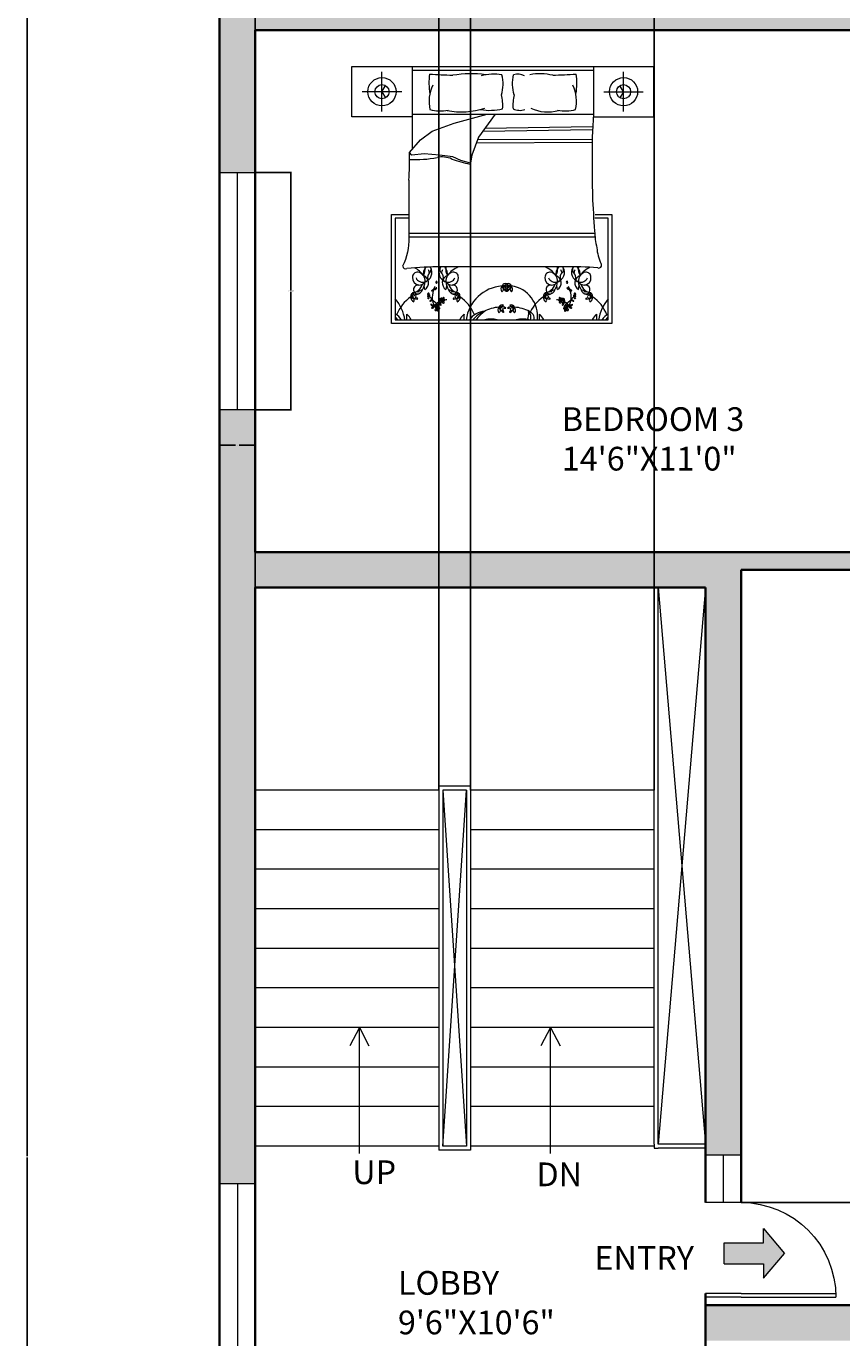
# Model space of a CAD drawing. Units: inches. Extents: x -26 to 13070, y -956 to 6917.
# Tile 6 of 13: x -26 to 180, y -466 to -134. Entities that reach past the tile are written whole.
import ezdxf

# ---------------------------------------------------------------- set-up
doc = ezdxf.new("R2010")
doc.units = ezdxf.units.IN
doc.header["$MEASUREMENT"] = 0
for name, color, linetype, lineweight in [('A-ANNO-DIMS', 2, 'Continuous', 18), ('A-ANNO-SYMB', 7, 'Continuous', 18), ('A-ANNO-TEXT', 7, 'Continuous', 18), ('A-AREA-IDEN', 7, 'Continuous', 18), ('A-DOOR', 3, 'Continuous', 18), ('A-FLOR-STRS', 7, 'Continuous', 18), ('A-FURN', 8, 'Continuous', 13), ('A-GLAZ', 4, 'Continuous', 18), ('A-WALL', 7, 'Continuous', 35), ('A-WALL-PATT', 252, 'Continuous', 13)]:
    doc.layers.add(name, color=color, linetype=linetype, lineweight=lineweight)
doc.styles.get("Standard").update_dxf_attribs({"font": 'arial.ttf'})
doc.dimstyles.get("Standard").update_dxf_attribs({"dimtxt": 0.18, "dimasz": 0.18, "dimexe": 0.18, "dimexo": 0.0625, "dimgap": 0.09, "dimtad": 0, "dimtih": 1, "dimtoh": 1, "dimdec": 0, "dimzin": 0, "dimdsep": 46, "dimlunit": 3, "dimtxsty": 'Standard', "dimcen": 0.09, "dimadec": 0, "dimazin": 0, "dimtfac": 1, "dimtdec": 0, "dimtofl": 0, "dimtmove": 0, "dimatfit": 3, "dimfxl": 1, "dimtolj": 1, "dimtzin": 0, "dimarcsym": 0})

# ---------------------------------------------------------------- blocks, each defined once
blk = doc.blocks.new('BED-DOUBLE-NIGHTSTANDS')
for p, q in [((0, 65), (76.43, 65)), ((7.64, 53.64), (7.64, 63.62)), ((15.29, 65), (15.29, 44.02)), ((61.14, 64.02), (15.29, 64.02)), ((68.79, 53.64), (68.79, 63.62)), ((12.64, 58.63), (2.65, 58.63)), ((63.79, 58.63), (73.78, 58.63)), ((15.29, 52.92), (61.14, 52.92)), ((20.33, 48.64), (25.9, 50.65)), ((25.9, 50.65), (34.24, 52.92)), ((36.28, 52.92), (32.09, 47.09)), ((14.6, 43.22), (17.39, 46.47)), ((17.39, 46.47), (20.33, 48.64)), ((32.09, 47.09), (30.39, 42.6)), ((60.87, 46.55), (31.85, 46.44)), ((60.91, 48.96), (33.16, 48.57)), ((60.94, 49.74), (33.73, 49.36)), ((15.22, 42.6), (14.6, 43.22)), ((60.87, 45.77), (31.55, 45.65)), ((18.32, 42.91), (15.22, 42.6)), ((22.19, 42.6), (18.32, 42.91)), ((25.59, 42.14), (22.19, 42.6)), ((27.6, 41.21), (25.59, 42.14)), ((30.08, 40.59), (27.6, 41.21)), ((30.39, 42.6), (30.08, 40.59)), ((10.09, 27.53), (14.41, 27.53)), ((10.09, 0), (10.09, 27.53)), ((14.41, 26.65), (10.97, 26.65)), ((10.97, 26.65), (10.97, 0.89)), ((64.92, 26.65), (61.55, 26.65)), ((61.57, 27.53), (65.81, 27.53)), ((64.92, 0.89), (64.92, 26.65)), ((65.81, 27.53), (65.81, 0)), ((61.56, 21.81), (14.4, 21.81)), ((61.49, 22.77), (14.41, 22.77)), ((53.73, 14.3), (22.7, 14.3)), ((18.51, 8.63), (18.34, 9.5)), ((23.85, 8.63), (24.02, 9.5)), ((52.05, 8.63), (51.88, 9.5)), ((57.39, 8.63), (57.56, 9.5)), ((10.97, 0.89), (64.92, 0.89)), ((65.81, 0), (10.09, 0))]:
    blk.add_line(p, q)
for points in [[(15.29, 52.26), (0, 52.26), (0, 65)], [(61.14, 65), (61.14, 52.26), (76.43, 52.26), (76.43, 65)], [(7.64, 58.63), (8.53, 60.17)], [(68.79, 58.63), (67.89, 60.17)], [(7.64, 58.63), (8.53, 57.08)], [(68.79, 58.63), (67.89, 57.08)]]:
    blk.add_lwpolyline(points)
for points in [[(19.68, 63.09, 0.074897), (19.77, 58.1, -0.472817)], [(56.75, 63.09, -0.074897), (56.66, 58.1, 0.472817)], [(37.86, 57.82, 0.14099), (38.01, 62.91, 0.235245)], [(41.12, 57.82, -0.14099), (40.97, 62.91, -0.235245)], [(14.44, 36.22, 0.001242), (14.4, 21.72, -0.127202), (12.87, 14.5)], [(61.47, 23.37, 0.056112), (62.02, 19.16, 0.095341), (63.1, 15.11)]]:
    blk.add_lwpolyline(points, format="xyb")
for centre, radius in [((7.64, 58.63), 3.57), ((7.64, 58.63), 1.78), ((68.79, 58.63), 3.57), ((68.79, 58.63), 1.78), ((21.65, 3.81), 0.195), ((22.92, 5.86), 0.195), ((52.98, 5.86), 0.195), ((54.25, 3.81), 0.195)]:
    blk.add_circle(centre, radius)
for centre, radius, start, end in [((61.8, 790.45), 728.57, 266.68521, 267.14978), ((30.15, 35.44), 27.72, 82.2196, 99.497), ((36, 49.44), 13.62, 81.5249, 103.96), ((42.02, 59.28), 3.78, 63.3437, 106.1026), ((47.68, 49.72), 13.44, 76.3427, 101.1841), ((14.63, 790.45), 728.57, 272.85022, 273.31479), ((29.41, 56.1), 9.85, 155.1316, 191.7583), ((47.02, 56.1), 9.85, 348.2417, 24.8684), ((28.85, 55.27), 9.36, 354.0129, 15.8293), ((50.13, 55.27), 9.36, 164.1707, 185.9871), ((22.4, 63.99), 10.24, 255.1039, 281.0369), ((27.79, 71.27), 17.76, 258.0397, 289.2615), ((34.99, 67.39), 13.48, 259.8617, 283.6238), ((42.53, 57.96), 4.05, 245.0183, 288.5407), ((49.61, 63.23), 9.73, 243.8761, 286.1746), ((54.03, 63.99), 10.24, 258.9631, 284.8961), ((198.16, 43.58), 137.33, 176.1, 180.9282), ((-55.48, 41.32), 70.1, 355.8294, 1.553), ((15.91, 70.29), 28.85, 267.4519, 281.3392), ((22.8, 35.91), 6.22, 66.2616, 101.3392), ((35.39, 69.47), 29.64, 250.1194, 259.3383), ((29.91, 40.53), 0.184, 268.8623, 19.7536), ((239.96, 38.59), 179.14, 179.1145, 184.8735), ((13.58, 14.54), 0.705, 183.98, 297.3412), ((21.79, -65.25), 79.56, 89.3433, 95.6887), ((13.28, 8.92), 5.78, 33.6671, 63.2997), ((21.03, 12.36), 2.95, 145.785, 184.7304), ((15.4, 13.74), 3.17, 328.8218, 9.1554), ((19.32, 13.46), 0.92, 120.0293, 142.325), ((17.85, 12.92), 2.44, 289.2822, 29.1751), ((17.48, 12.48), 2.2, 7.436, 29.9149), ((18.93, 13.64), 1.14, 311.5653, 23.8354), ((19.32, 13.46), 0.92, 44.4517, 63.558), ((24.5, 12.92), 2.44, 150.8249, 250.7178), ((23.42, 13.64), 1.14, 156.1646, 228.4347), ((23.03, 13.46), 0.92, 113.229, 135.5483), ((24.87, 12.48), 2.2, 150.0851, 172.564), ((23.03, 13.46), 0.92, 37.675, 66.7144), ((21.32, 12.36), 2.95, 355.2696, 34.215), ((26.95, 13.74), 3.17, 169.7133, 211.1782), ((29.07, 8.92), 5.78, 111.4941, 146.3329), ((46.82, 8.92), 5.78, 33.6671, 68.5059), ((54.57, 12.36), 2.95, 145.785, 184.7304), ((48.94, 13.74), 3.17, 328.8218, 10.2867), ((52.87, 13.46), 0.92, 113.2856, 142.325), ((51.4, 12.92), 2.44, 289.2822, 29.1751), ((51.03, 12.48), 2.2, 7.436, 29.9149), ((52.87, 13.46), 0.92, 44.4517, 66.7144), ((52.48, 13.64), 1.14, 311.5653, 23.8354), ((56.07, -60.03), 74.37, 85.2402, 91.8035), ((58.04, 12.92), 2.44, 150.8249, 250.7178), ((56.96, 13.64), 1.14, 156.1646, 228.4347), ((56.57, 13.46), 0.92, 106.6343, 135.5483), ((58.41, 12.48), 2.2, 150.0851, 172.564), ((56.57, 13.46), 0.92, 37.675, 72.5814), ((54.87, 12.36), 2.95, 355.2696, 34.215), ((60.5, 13.74), 3.17, 169.249, 211.1782), ((62.62, 8.92), 5.78, 113.6453, 146.3329), ((62.52, 14.72), 0.697, 246.5219, 33.8264), ((17.18, 11.52), 1.83, 174.9449, 262.8857), ((16.65, 11.7), 1.29, 84.4856, 181.0538), ((17.9, 12.21), 1.77, 201.5819, 291.4221), ((14.48, 11.1), 3.61, 301.2614, 341.7045), ((16.25, 10.75), 2.3, 355.2933, 76.921), ((16.86, 11.92), 2.22, 272.3591, 324.0401), ((14.45, 10.81), 4.1, 326.2883, 356.5076), ((17.56, 10.28), 1.9, 299.9085, 73.1337), ((21.03, 12.36), 2.95, 212.7011, 216.3445), ((18.76, 11.08), 0.474, 257.3041, 15.1471), ((20.73, 11.61), 1.57, 131.5653, 195.1471), ((21.4, 10.36), 0.147, 102.7051, 280.4384), ((21.38, 10.45), 0.24, 280.4384, 100.4136), ((21.62, 11.61), 1.57, 344.8529, 48.4347), ((24.79, 10.28), 1.9, 106.8663, 240.0915), ((23.59, 11.08), 0.474, 164.8529, 282.6959), ((21.32, 12.36), 2.95, 323.6555, 327.2989), ((25.49, 11.92), 2.22, 215.9599, 267.6409), ((26.1, 10.75), 2.3, 103.079, 184.7067), ((24.46, 12.21), 1.77, 248.5779, 338.4181), ((27.9, 10.81), 4.1, 183.4924, 213.7117), ((27.87, 11.1), 3.61, 198.2955, 238.7386), ((25.17, 11.52), 1.83, 277.1143, 5.0551), ((25.7, 11.7), 1.29, 358.9462, 95.5144), ((38.83, 9.26), 0.827, 63.0274, 163.8037), ((37.99, 11.2), 1.7, 271.4585, 315.3727), ((39.62, 9.26), 0.827, 16.1963, 116.9726), ((40.45, 11.2), 1.7, 224.6273, 268.5415), ((50.72, 11.52), 1.83, 174.9449, 262.8857), ((50.19, 11.7), 1.29, 84.4856, 181.0538), ((51.44, 12.21), 1.77, 201.5819, 291.4221), ((48.03, 11.1), 3.61, 301.2614, 341.7045), ((49.8, 10.75), 2.3, 355.2933, 76.921), ((50.4, 11.92), 2.22, 272.3591, 324.0401), ((47.99, 10.81), 4.1, 326.2883, 356.5076), ((51.1, 10.28), 1.9, 299.9085, 73.1337), ((54.57, 12.36), 2.95, 212.7011, 216.3445), ((52.3, 11.08), 0.474, 257.3041, 15.1471), ((54.28, 11.61), 1.57, 131.5653, 195.1471), ((54.52, 10.45), 0.24, 79.5864, 259.5616), ((54.5, 10.36), 0.147, 259.5616, 77.2949), ((55.16, 11.61), 1.57, 344.8529, 48.4347), ((58.34, 10.28), 1.9, 106.8663, 240.0915), ((57.13, 11.08), 0.474, 164.8529, 282.6959), ((54.87, 12.36), 2.95, 323.6555, 327.2989), ((59.04, 11.92), 2.22, 215.9599, 267.6409), ((59.64, 10.75), 2.3, 103.079, 184.7067), ((58, 12.21), 1.77, 248.5779, 338.4181), ((61.45, 10.81), 4.1, 183.4924, 213.7117), ((61.41, 11.1), 3.61, 198.2955, 238.7386), ((58.72, 11.52), 1.83, 277.1143, 5.0551), ((59.25, 11.7), 1.29, 358.9462, 95.5144), ((20.62, -1.45), 9.98, 124.3865, 158.5908), ((15.79, 6.99), 0.827, 92.9516, 193.728), ((16.06, 6.55), 1.11, 167.7115, 249.0387), ((14.09, 8.25), 1.7, 301.3827, 345.2969), ((16.26, 5.87), 1.58, 75.4653, 144.2343), ((13.47, 13.61), 6.98, 282.5173, 297.1824), ((14.96, 5.96), 0.834, 328.4633, 88.2869), ((16.64, 8.69), 2.52, 228.8402, 267.9352), ((15.7, 7.17), 0.816, 207.6827, 313.7762), ((16.76, 8.57), 1.15, 80.264, 250.8688), ((16.52, 7.33), 0.703, 63.9755, 143.2681), ((16.19, 6.66), 0.108, 313.7762, 249.7183), ((16.48, 8.92), 1.43, 265.969, 344.3045), ((18.02, 7.01), 1.53, 96.1662, 141.5825), ((19.42, 7.32), 0.325, 101.5637, 142.6358), ((19.15, 7.02), 0.195, 273.2768, 86.7232), ((19.37, 7.21), 0.186, 91.1081, 181.8675), ((19.76, 7.09), 0.591, 203.4276, 227.6104), ((19.57, 6.83), 0.402, 80.3487, 133.6538), ((19.5, 7.16), 0.318, 229.7889, 317.6792), ((19.16, 7.58), 0.468, 288.7263, 352.5032), ((19.14, 6.49), 0.452, 355.053, 68.3618), ((19.5, 6.41), 0.637, 83.0852, 105.7171), ((19.47, 7.55), 0.15, 345.2356, 144.9248), ((15.08, 1.13), 7.26, 43.1541, 52.0459), ((19.61, 7.06), 0.168, 317.6792, 80.3487), ((20.55, 8.08), 0.401, 101.3256, 154.4621), ((19.97, 9.45), 1.21, 280.2588, 300.656), ((20.25, 10.41), 2.16, 268.3264, 277.1302), ((26.69, 6.51), 6.33, 163.5842, 183.8277), ((19.71, 9.44), 1.23, 308.2101, 316.3071), ((20.47, 8.64), 0.367, 278.3432, 4.2869), ((20.26, 8.96), 0.641, 300.656, 332.6341), ((20.74, 8.53), 0.156, 55.7657, 157.4417), ((26.69, 6.51), 6.33, 153.0032, 159.8941), ((20.99, 8.68), 0.156, 84.3784, 186.0543), ((20.84, 9.3), 0.641, 269.1859, 301.164), ((21.03, 8.97), 0.367, 237.5332, 323.4768), ((20.67, 10.02), 1.23, 285.5129, 293.6099), ((20.55, 9.79), 1.21, 301.164, 321.5612), ((21.48, 8.64), 0.401, 87.3579, 140.4944), ((19.56, 10), 2.16, 324.6898, 333.4936), ((24.33, 7.01), 1.53, 38.4175, 83.8338), ((25.87, 8.92), 1.43, 195.6955, 274.031), ((25.59, 8.57), 1.15, 289.1312, 99.736), ((25.83, 7.33), 0.703, 36.7319, 116.0245), ((26.09, 5.87), 1.58, 35.7657, 104.5347), ((28.88, 13.61), 6.98, 242.8176, 257.4827), ((25.71, 8.69), 2.52, 272.0648, 311.1598), ((26.65, 7.17), 0.816, 226.2238, 332.3173), ((26.17, 6.7), 0.0651, 290.2667, 226.2271), ((27.4, 5.96), 0.834, 91.7131, 211.5367), ((26.57, 6.99), 0.827, 346.272, 87.0484), ((28.26, 8.25), 1.7, 194.7031, 238.6173), ((26.29, 6.55), 1.11, 290.9613, 12.2885), ((21.73, -1.45), 9.98, 21.4092, 55.6135), ((38.81, -0.46), 9.98, 94.4623, 172.255), ((38.85, 8.75), 1.11, 137.7873, 219.1145), ((37.6, 8.78), 0.834, 298.5391, 58.3627), ((38.68, 8.05), 1.58, 45.5411, 114.3101), ((40.12, 16.15), 6.98, 252.593, 267.2582), ((38.85, 9.46), 0.816, 177.7585, 283.852), ((40.42, 10.31), 2.52, 198.9159, 238.011), ((39.76, 8.05), 1.58, 65.6899, 134.4589), ((38.32, 16.15), 6.98, 272.7418, 287.407), ((39.02, 8.77), 0.108, 283.852, 219.9245), ((39.15, 8.27), 0.124, 238.011, 71.5592), ((39.17, 8.33), 0.0602, 71.5592, 188.0167), ((39.29, 8.27), 0.124, 108.4408, 301.989), ((39.27, 8.33), 0.0602, 351.9833, 108.4408), ((39.42, 8.81), 0.0651, 320.1909, 256.0209), ((38.02, 10.31), 2.52, 301.989, 341.0841), ((39.6, 9.46), 0.816, 256.148, 2.2415), ((40.85, 8.78), 0.834, 121.6373, 241.4609), ((39.59, 8.75), 1.11, 320.8855, 42.2127), ((39.31, 1.85), 7.72, 352.8636, 81.8197), ((54.16, -1.45), 9.98, 124.3865, 158.5908), ((49.33, 6.99), 0.827, 92.9516, 193.728), ((49.61, 6.55), 1.11, 167.7115, 249.0387), ((47.64, 8.25), 1.7, 301.3827, 345.2969), ((49.81, 5.87), 1.58, 75.4653, 144.2343), ((47.01, 13.61), 6.98, 282.5173, 297.1824), ((49.25, 7.17), 0.816, 207.6827, 313.7762), ((50.19, 8.69), 2.52, 228.8402, 267.9352), ((48.5, 5.96), 0.834, 328.4633, 88.2869), ((50.3, 8.57), 1.15, 80.264, 250.8688), ((50.06, 7.33), 0.703, 63.9755, 143.2681), ((49.74, 6.66), 0.108, 313.7762, 249.7183), ((50.03, 8.92), 1.43, 265.969, 344.3045), ((51.57, 7.01), 1.53, 96.1662, 141.5825), ((55.35, 9.79), 1.21, 218.4388, 238.836), ((54.42, 8.64), 0.401, 39.5056, 92.6421), ((56.33, 10), 2.16, 206.5064, 215.3102), ((54.87, 8.97), 0.367, 216.5232, 302.4668), ((55.05, 9.3), 0.641, 238.836, 270.8141), ((55.22, 10.02), 1.23, 246.3901, 254.4871), ((49.2, 6.51), 6.33, 20.1059, 26.9968), ((54.91, 8.68), 0.156, 353.9457, 95.6216), ((55.15, 8.53), 0.156, 22.5583, 124.2343), ((55.43, 8.64), 0.367, 175.7131, 261.6568), ((55.63, 8.96), 0.641, 207.3659, 239.344), ((49.2, 6.51), 6.33, 356.1723, 16.4158), ((56.18, 9.44), 1.23, 223.6929, 231.7899), ((55.92, 9.45), 1.21, 239.344, 259.7412), ((55.64, 10.41), 2.16, 262.8698, 271.6736), ((55.34, 8.08), 0.401, 25.5379, 78.6744), ((60.81, 1.13), 7.26, 127.9541, 136.8459), ((56.28, 7.06), 0.168, 99.6513, 222.3208), ((56.4, 7.16), 0.318, 222.3208, 310.2111), ((56.32, 6.83), 0.402, 46.3462, 99.6513), ((56.42, 7.55), 0.15, 35.0752, 194.7644), ((56.74, 7.58), 0.468, 187.4968, 251.2737), ((56.76, 6.49), 0.452, 111.6382, 184.947), ((56.4, 6.41), 0.637, 74.2829, 96.9148), ((56.52, 7.21), 0.186, 358.1325, 88.8919), ((56.14, 7.09), 0.591, 312.3896, 336.5724), ((56.48, 7.32), 0.325, 37.3642, 78.4363), ((56.75, 7.02), 0.195, 93.2768, 266.7232), ((59.41, 8.92), 1.43, 195.6955, 274.031), ((57.87, 7.01), 1.53, 38.4175, 83.8338), ((59.14, 8.57), 1.15, 289.1312, 99.736), ((59.37, 7.33), 0.703, 36.7319, 116.0245), ((59.63, 5.87), 1.58, 35.7657, 104.5347), ((62.43, 13.61), 6.98, 242.8176, 257.4827), ((59.25, 8.69), 2.52, 272.0648, 311.1598), ((60.19, 7.17), 0.816, 226.2238, 332.3173), ((59.71, 6.7), 0.0651, 290.2667, 226.2271), ((60.94, 5.96), 0.834, 91.7131, 211.5367), ((61.8, 8.25), 1.7, 194.7031, 238.6173), ((60.11, 6.99), 0.827, 346.272, 87.0484), ((59.83, 6.55), 1.11, 290.9613, 12.2885), ((55.28, -1.45), 9.98, 21.4092, 55.6135), ((3.54, -0.46), 9.98, 7.745, 41.8856), ((16.54, 6.35), 0.0602, 101.4834, 217.9409), ((16.56, 6.29), 0.124, 267.9352, 101.4834), ((19.41, 6.66), 0.321, 217.7621, 259.0403), ((19.44, 6.46), 0.149, 232.4737, 355.053), ((20.1, 5.51), 0.401, 101.3256, 154.4621), ((19.52, 6.87), 1.21, 280.2588, 300.656), ((19.8, 7.84), 2.16, 268.3264, 277.1302), ((20.23, 4.81), 0.217, 146.8636, 236.9021), ((19.26, 6.87), 1.23, 308.2101, 316.3071), ((23.3, 9.6), 5.69, 235.1882, 238.8844), ((20.6, 5.12), 0.588, 199.4799, 267.6828), ((20.01, 6.06), 0.367, 278.3432, 4.2869), ((20.54, 4.9), 0.507, 212.8155, 277.3992), ((19.81, 6.39), 0.641, 300.656, 332.6341), ((20.29, 5.96), 0.156, 55.7657, 157.4417), ((20.24, 4.56), 0.588, 266.9701, 338.2913), ((17.14, 8.76), 5.69, 302.6784, 306.3746), ((20.39, 4.1), 0.217, 214.3538, 304.3923), ((20.47, 4.92), 0.225, 238.8844, 314.2646), ((23.54, 6.35), 3.17, 184.756, 209.2041), ((28.11, 13.11), 10.44, 222.2412, 232.1744), ((20.42, 4.42), 0.507, 280.3057, 17.1958), ((20.38, 4.36), 0.225, 306.3746, 21.7548), ((20.75, 4.51), 0.17, 19.3605, 201.7548), ((20.75, 4.64), 0.17, 311.8703, 134.2646), ((23.94, 3.09), 3.39, 153.7819, 158.2913), ((21.24, 5.41), 0.887, 247.2305, 319.0635), ((20.95, 5.11), 0.522, 264.4544, 310.6188), ((23.54, 6.35), 3.17, 214.0033, 222.4917), ((21.33, 4.9), 0.539, 218.3208, 298.8162), ((23.87, 2.14), 3.81, 120.544, 139.818), ((21.24, 3.45), 0.193, 148.0499, 225.6268), ((21.6, 3.23), 0.614, 104.7558, 148.0499), ((21.25, 3.66), 0.384, 247.4086, 351.4386), ((21.43, 4.08), 0.265, 126.1046, 271.4281), ((21.4, 4.16), 0.191, 353.7526, 131.7054), ((21.7, 4.23), 0.628, 70.0041, 130.6188), ((21.36, 3.65), 0.129, 262.906, 7.132), ((21.22, 3.93), 0.268, 0.0645, 61.1507), ((21.29, 4.16), 0.306, 311.8413, 355.7877), ((21.29, 5), 0.645, 297.7043, 344.3516), ((21.92, 4.11), 0.325, 101.5637, 176.365), ((21.91, 3.45), 0.321, 151.2196, 259.0403), ((21.87, 4), 0.186, 91.1081, 181.8675), ((22.26, 3.88), 0.591, 203.4276, 227.6104), ((22.07, 3.62), 0.402, 80.3487, 133.6538), ((22, 3.96), 0.318, 229.7889, 317.6792), ((21.66, 4.37), 0.468, 288.7263, 352.5032), ((21.64, 3.28), 0.452, 355.053, 68.3618), ((22, 3.21), 0.637, 83.0852, 105.7171), ((21.97, 4.35), 0.15, 345.2356, 144.9248), ((21.43, 6.15), 0.887, 304.5369, 16.3699), ((21.9, 5.96), 0.539, 272.8499, 356.1226), ((21.52, 5.75), 0.522, 321.7607, 7.9252), ((21.63, 5), 0.522, 8.7227, 54.8872), ((21.66, 4.58), 0.887, 0.278, 72.111), ((22.66, 5.9), 0.628, 127.3105, 187.9252), ((22.06, 4.9), 0.539, 20.5253, 88.5375), ((22.11, 3.85), 0.168, 317.6792, 80.3487), ((22.77, 5.17), 0.628, 188.7227, 249.3375), ((21.8, 5.98), 0.645, 355.0106, 41.658), ((22.51, 5.5), 0.193, 148.0499, 225.6268), ((23.87, 2.14), 3.81, 113.0501, 113.8477), ((22.87, 5.28), 0.614, 104.7558, 148.0499), ((22.52, 5.72), 0.384, 247.4086, 351.4386), ((22.71, 6.14), 0.265, 126.1046, 271.4281), ((22.68, 6.21), 0.191, 353.7526, 131.7054), ((21.96, 4.86), 0.645, 334.9899, 21.6373), ((22.63, 5.7), 0.129, 262.906, 7.132), ((22.5, 5.98), 0.268, 0.0645, 61.1507), ((22.56, 6.21), 0.306, 311.8413, 355.7877), ((23.19, 5.5), 0.321, 151.2196, 259.0403), ((23.19, 6.17), 0.325, 101.5637, 176.365), ((23.15, 6.05), 0.186, 91.1081, 181.8675), ((23.53, 5.93), 0.591, 203.4276, 227.6104), ((23.35, 5.67), 0.402, 80.3487, 133.6538), ((23.27, 6.01), 0.318, 229.7889, 317.6792), ((22.93, 6.42), 0.468, 288.7263, 352.5032), ((22.91, 5.33), 0.452, 355.053, 68.3618), ((23.27, 5.26), 0.637, 83.0852, 105.7171), ((23.25, 6.4), 0.15, 345.2356, 144.9248), ((23.22, 5.31), 0.149, 232.4737, 355.053), ((23.38, 5.91), 0.168, 317.6792, 80.3487), ((23.87, 2.14), 3.81, 87.1071, 94.7585), ((25.8, 6.29), 0.124, 78.5166, 272.0648), ((25.81, 6.35), 0.0602, 322.0591, 78.5166), ((38.04, -5.81), 9.98, 94.4623, 117.4146), ((38.09, 3.4), 1.11, 137.7873, 219.1145), ((36.83, 3.44), 0.834, 298.5391, 58.3627), ((38.06, 3.91), 0.827, 63.0274, 163.8037), ((37.22, 5.85), 1.7, 271.4585, 315.3727), ((37.92, 2.71), 1.58, 45.5411, 114.3101), ((39.66, 4.96), 2.52, 198.9159, 238.011), ((39.36, 10.81), 6.98, 252.593, 267.2582), ((38.08, 4.11), 0.816, 177.7585, 283.852), ((38.25, 3.43), 0.108, 283.852, 219.9245), ((40.53, 2.71), 1.58, 65.6899, 134.4589), ((39.09, 10.81), 6.98, 272.7418, 287.407), ((40.38, 3.91), 0.827, 16.1963, 116.9726), ((41.22, 5.85), 1.7, 224.6273, 268.5415), ((40.18, 3.47), 0.0651, 320.1909, 256.0209), ((38.79, 4.96), 2.52, 301.989, 341.0841), ((40.36, 4.11), 0.816, 256.148, 2.2415), ((41.61, 3.44), 0.834, 121.6373, 241.4609), ((40.36, 3.4), 1.11, 320.8855, 42.2127), ((40.4, -5.81), 9.98, 62.5854, 85.5377), ((50.09, 6.35), 0.0602, 101.4834, 217.9409), ((50.1, 6.29), 0.124, 267.9352, 101.4834), ((52.03, 2.14), 3.81, 85.2415, 92.8929), ((52.51, 5.91), 0.168, 99.6513, 222.3208), ((52.62, 6.01), 0.318, 222.3208, 310.2111), ((52.55, 5.67), 0.402, 46.3462, 99.6513), ((52.65, 6.4), 0.15, 35.0752, 194.7644), ((52.97, 6.42), 0.468, 187.4968, 251.2737), ((52.98, 5.33), 0.452, 111.6382, 184.947), ((52.68, 5.31), 0.149, 184.947, 307.5263), ((52.63, 5.26), 0.637, 74.2829, 96.9148), ((52.75, 6.05), 0.186, 358.1325, 88.8919), ((52.36, 5.93), 0.591, 312.3896, 336.5724), ((52.71, 6.17), 0.325, 3.635, 78.4363), ((52.71, 5.5), 0.321, 280.9597, 28.7804), ((53.37, 5.72), 0.384, 188.5614, 292.5914), ((53.22, 6.21), 0.191, 48.2946, 186.2474), ((53.34, 6.21), 0.306, 184.2123, 228.1587), ((53.4, 5.98), 0.268, 118.8493, 179.9355), ((53.26, 5.7), 0.129, 172.868, 277.094), ((53.19, 6.14), 0.265, 268.5719, 53.8954), ((53.03, 5.28), 0.614, 31.9501, 75.2442), ((53.93, 4.86), 0.645, 158.3627, 205.0101), ((53.84, 4.9), 0.539, 91.4625, 159.4747), ((54.23, 4.58), 0.887, 107.889, 179.722), ((53.13, 5.17), 0.628, 290.6625, 351.2773), ((54.1, 5.98), 0.645, 138.342, 184.9894), ((53.99, 5.96), 0.539, 183.8774, 267.1501), ((52.03, 2.14), 3.81, 66.1523, 66.9499), ((53.38, 5.5), 0.193, 314.3732, 31.9501), ((54.47, 6.15), 0.887, 163.6301, 235.4631), ((53.23, 5.9), 0.628, 352.0748, 52.6895), ((53.78, 3.85), 0.168, 99.6513, 222.3208), ((53.9, 3.96), 0.318, 222.3208, 310.2111), ((54.26, 5), 0.522, 125.1128, 171.2773), ((53.82, 3.62), 0.402, 46.3462, 99.6513), ((53.92, 4.35), 0.15, 35.0752, 194.7644), ((54.24, 4.37), 0.468, 187.4968, 251.2737), ((54.26, 3.28), 0.452, 111.6382, 184.947), ((53.9, 3.21), 0.637, 74.2829, 96.9148), ((54.37, 5.75), 0.522, 172.0748, 218.2393), ((52.03, 2.14), 3.81, 40.182, 59.456), ((54.2, 4.23), 0.628, 49.3812, 109.9959), ((54.65, 5.41), 0.887, 220.9365, 292.7695), ((54.6, 5), 0.645, 195.6484, 242.2957), ((54.02, 4), 0.186, 358.1325, 88.8919), ((53.64, 3.88), 0.591, 312.3896, 336.5724), ((53.98, 4.11), 0.325, 3.635, 78.4363), ((53.98, 3.45), 0.321, 280.9597, 28.7804), ((47.79, 13.11), 10.44, 307.8256, 317.7588), ((54.64, 3.66), 0.384, 188.5614, 292.5914), ((54.56, 4.9), 0.539, 241.1838, 321.6792), ((54.49, 4.16), 0.191, 48.2946, 186.2474), ((54.61, 4.16), 0.306, 184.2123, 228.1587), ((54.67, 3.93), 0.268, 118.8493, 179.9355), ((54.54, 3.65), 0.129, 172.868, 277.094), ((54.46, 4.08), 0.265, 268.5719, 53.8954), ((54.3, 3.23), 0.614, 31.9501, 75.2442), ((54.95, 5.11), 0.522, 229.3812, 275.5456), ((52.36, 6.35), 3.17, 317.5083, 325.9967), ((54.66, 3.45), 0.193, 314.3732, 31.9501), ((55.47, 4.42), 0.507, 162.8042, 259.6943), ((55.15, 4.64), 0.17, 45.7354, 228.1297), ((55.15, 4.51), 0.17, 338.2452, 160.6395), ((51.96, 3.09), 3.39, 21.7087, 26.2181), ((55.65, 4.56), 0.588, 201.7087, 273.0299), ((52.36, 6.35), 3.17, 330.7959, 355.244), ((55.42, 4.92), 0.225, 225.7354, 301.1156), ((55.36, 4.9), 0.507, 262.6008, 327.1845), ((55.51, 4.36), 0.225, 158.2452, 233.6254), ((55.29, 5.12), 0.588, 272.3172, 340.5201), ((58.75, 8.76), 5.69, 233.6254, 237.3216), ((55.5, 4.1), 0.217, 235.6077, 325.6462), ((55.61, 5.96), 0.156, 22.5583, 124.2343), ((55.88, 6.06), 0.367, 175.7131, 261.6568), ((56.09, 6.39), 0.641, 207.3659, 239.344), ((52.6, 9.6), 5.69, 301.1156, 304.8118), ((56.64, 6.87), 1.23, 223.6929, 231.7899), ((56.38, 6.87), 1.21, 239.344, 259.7412), ((55.66, 4.81), 0.217, 303.0979, 33.1364), ((56.1, 7.84), 2.16, 262.8698, 271.6736), ((55.8, 5.51), 0.401, 25.5379, 78.6744), ((56.45, 6.46), 0.149, 184.947, 307.5263), ((56.48, 6.66), 0.321, 280.9597, 322.2379), ((59.34, 6.29), 0.124, 78.5166, 272.0648), ((59.35, 6.35), 0.0602, 322.0591, 78.5166), ((72.35, -0.46), 9.98, 138.1144, 172.255), ((8.55, -1.8), 4.86, 33.4617, 60.1116), ((6.8, -2.7), 6.06, 36.3036, 46.4814), ((11.27, -0.67), 4.06, 22.5547, 48.9546), ((0.16, 1.51), 13.81, 357.4081, 3.6519), ((21.94, 3.26), 0.149, 232.4737, 355.053), ((31.08, -0.67), 4.06, 131.0454, 157.4453), ((42.19, 1.51), 13.81, 176.3481, 182.5919), ((33.8, -1.8), 4.86, 91.272, 146.5383), ((35.55, -2.7), 6.06, 107.8504, 143.6964), ((38.74, -4.41), 9.02, 124.0123, 144.053), ((35.25, -4.36), 5.49, 73.5431, 107.0202), ((37.43, -7.19), 8.12, 94.3787, 95.6357), ((41.7, -12.75), 14.5, 109.7217, 109.9028), ((38.38, 2.93), 0.124, 238.011, 71.5592), ((38.4, 2.99), 0.0602, 71.5592, 188.0167), ((40.06, 2.93), 0.124, 108.4408, 301.989), ((40.04, 2.99), 0.0602, 351.9833, 108.4408), ((43.19, -4.36), 5.49, 72.9798, 106.4569), ((41.02, -7.19), 8.12, 84.3643, 85.6213), ((36.74, -12.75), 14.5, 70.0972, 70.2783), ((40.31, 2.55), 4.47, 338.117, 6.6195), ((44.41, 1.31), 1.79, 346.3898, 79.0739), ((43.06, 1.55), 2.27, 342.8609, 41.9049), ((33.7, 1.51), 13.81, 357.4081, 3.6519), ((44.82, -0.67), 4.06, 22.5547, 48.9546), ((53.95, 3.26), 0.149, 184.947, 307.5263), ((64.62, -0.67), 4.06, 131.0454, 157.4453), ((75.74, 1.51), 13.81, 176.3481, 182.5919), ((67.35, -1.8), 4.86, 119.8884, 146.5383), ((69.1, -2.7), 6.06, 133.5186, 143.6964)]:
    blk.add_arc(centre, radius, start, end)
blk = doc.blocks.new('DOOR-SWING-24')
for p, q in [((24, 1), (0, 1)), ((24, 0), (0, 0))]:
    blk.add_line(p, q)
blk.add_arc((24, 0), 24, 90, 180)
blk = doc.blocks.new('WIN-60')
for p, q in [((0, 0), (0, 60)), ((0, 60), (9, 60)), ((4.5, 0), (4.5, 60)), ((9, 60), (9, 0)), ((9, 0), (0, 0))]:
    blk.add_line(p, q)
blk = doc.blocks.new('STAIR-TRAVEL-ARROW')
for p, q in [((2.41, 31.83), (0, 27.19)), ((2.41, 0), (2.41, 31.83)), ((2.41, 31.83), (4.82, 27.19))]:
    blk.add_line(p, q)
blk = doc.blocks.new('*D20')
at = {"layer": 'A-ANNO-DIMS', "color": 0, "lineweight": -2, "transparency": 16777216}
for p, q in [((31.7, -171.04), (40.82, -171.04)), ((40.64, -171.22), (40.64, -200.86)), ((40.64, -230.86), (40.64, -201.22)), ((31.7, -231.04), (40.82, -231.04))]:
    blk.add_line(p, q, dxfattribs=at)
at = {"layer": 'A-ANNO-DIMS', "color": 0, "transparency": 16777216}
for points in [[(40.61, -171.22), (40.67, -171.22), (40.64, -171.04)], [(40.61, -230.86), (40.67, -230.86), (40.64, -231.04)]]:
    blk.add_solid(points, dxfattribs=at)
at = {"layer": 'Defpoints', "color": 0, "transparency": 16777216}
for p in [(31.64, -171.04), (40.64, -171.04), (31.64, -231.04)]:
    blk.add_point(p, dxfattribs=at)
at = {"layer": 'A-ANNO-DIMS', "color": 0, "transparency": 16777216, "insert": (40.64, -201.04), "char_height": 0.18, "attachment_point": 5}
blk.add_mtext('\\A1;WINDOW 60 TYP.', dxfattribs=at)
blk = doc.blocks.new('*D21')
at = {"layer": 'A-ANNO-DIMS', "color": 0, "lineweight": -2, "transparency": 16777216}
for p, q in [((22.64, -231.1), (22.64, -240.22)), ((31.64, -231.1), (31.64, -240.22)), ((22.82, -240.04), (26.68, -240.04)), ((31.46, -240.04), (27.6, -240.04))]:
    blk.add_line(p, q, dxfattribs=at)
at = {"layer": 'A-ANNO-DIMS', "color": 0, "transparency": 16777216}
for points in [[(22.82, -240.01), (22.82, -240.07), (22.64, -240.04)], [(31.46, -240.01), (31.46, -240.07), (31.64, -240.04)]]:
    blk.add_solid(points, dxfattribs=at)
at = {"layer": 'Defpoints', "color": 0, "transparency": 16777216}
for p in [(22.64, -231.04), (31.64, -231.04), (31.64, -240.04)]:
    blk.add_point(p, dxfattribs=at)
at = {"layer": 'A-ANNO-DIMS', "color": 0, "transparency": 16777216, "insert": (27.14, -240.04), "char_height": 0.18, "attachment_point": 5}
blk.add_mtext('\\A1;9 TYP.', dxfattribs=at)
blk = doc.blocks.new('*D41')
at = {"layer": 'A-ANNO-DIMS', "color": 0, "lineweight": -2, "transparency": 16777216}
for p, q in [((214.58, 67.46), (-26.29, 67.46)), ((-26.11, 67.28), (-26.11, -419.86)), ((-26.11, -907.36), (-26.11, -420.22)), ((208.58, -907.54), (-26.29, -907.54))]:
    blk.add_line(p, q, dxfattribs=at)
at = {"layer": 'A-ANNO-DIMS', "color": 0, "transparency": 16777216}
for points in [[(-26.14, 67.28), (-26.08, 67.28), (-26.11, 67.46)], [(-26.14, -907.36), (-26.08, -907.36), (-26.11, -907.54)]]:
    blk.add_solid(points, dxfattribs=at)
at = {"layer": 'Defpoints', "color": 0, "transparency": 16777216}
for p in [(-26.11, 67.46), (214.64, 67.46), (208.64, -907.54)]:
    blk.add_point(p, dxfattribs=at)
at = {"layer": 'A-ANNO-DIMS', "color": 0, "transparency": 16777216, "insert": (-26.11, -420.04), "char_height": 0.18, "attachment_point": 5}
blk.add_mtext('\\A1;975', dxfattribs=at)
blk = doc.blocks.new('*D55')
at = {"layer": 'A-ANNO-DIMS', "color": 0, "lineweight": -2, "transparency": 16777216}
for p, q in [((31.64, -327.23), (31.64, 116.39)), ((31.82, 116.21), (54.56, 116.21)), ((77.96, 116.21), (55.22, 116.21)), ((78.14, -327.23), (78.14, 116.39))]:
    blk.add_line(p, q, dxfattribs=at)
at = {"layer": 'A-ANNO-DIMS', "color": 0, "transparency": 16777216}
for points in [[(31.82, 116.24), (31.82, 116.18), (31.64, 116.21)], [(77.96, 116.24), (77.96, 116.18), (78.14, 116.21)]]:
    blk.add_solid(points, dxfattribs=at)
at = {"layer": 'Defpoints', "color": 0, "transparency": 16777216}
for p in [(78.14, 116.21), (31.64, -327.29), (78.14, -327.29)]:
    blk.add_point(p, dxfattribs=at)
at = {"layer": 'A-ANNO-DIMS', "color": 0, "transparency": 16777216, "insert": (54.89, 116.21), "char_height": 0.18, "attachment_point": 5}
blk.add_mtext('\\A1;46.5', dxfattribs=at)
blk = doc.blocks.new('*D56')
at = {"layer": 'A-ANNO-DIMS', "color": 0, "lineweight": -2, "transparency": 16777216}
for p, q in [((86.14, -327.23), (86.14, 116.39)), ((86.32, 116.21), (109.06, 116.21)), ((132.46, 116.21), (109.72, 116.21)), ((132.64, -327.23), (132.64, 116.39))]:
    blk.add_line(p, q, dxfattribs=at)
at = {"layer": 'A-ANNO-DIMS', "color": 0, "transparency": 16777216}
for points in [[(86.32, 116.24), (86.32, 116.18), (86.14, 116.21)], [(132.46, 116.24), (132.46, 116.18), (132.64, 116.21)]]:
    blk.add_solid(points, dxfattribs=at)
at = {"layer": 'Defpoints', "color": 0, "transparency": 16777216}
for p in [(132.64, 116.21), (86.14, -327.29), (132.64, -327.29)]:
    blk.add_point(p, dxfattribs=at)
at = {"layer": 'A-ANNO-DIMS', "color": 0, "transparency": 16777216, "insert": (109.39, 116.21), "char_height": 0.18, "attachment_point": 5}
blk.add_mtext('\\A1;46.5', dxfattribs=at)
blk = doc.blocks.new('*D57')
at = {"layer": 'A-ANNO-DIMS', "color": 0, "lineweight": -2, "transparency": 16777216}
for p, q in [((154.7, -271.54), (596.57, -271.54)), ((596.39, -271.72), (596.39, -351.36)), ((596.39, -431.36), (596.39, -351.72)), ((154.7, -431.54), (596.57, -431.54))]:
    blk.add_line(p, q, dxfattribs=at)
at = {"layer": 'A-ANNO-DIMS', "color": 0, "transparency": 16777216}
for points in [[(596.36, -271.72), (596.42, -271.72), (596.39, -271.54)], [(596.36, -431.36), (596.42, -431.36), (596.39, -431.54)]]:
    blk.add_solid(points, dxfattribs=at)
at = {"layer": 'Defpoints', "color": 0, "transparency": 16777216}
for p in [(154.64, -271.54), (596.39, -271.54), (154.64, -431.54)]:
    blk.add_point(p, dxfattribs=at)
at = {"layer": 'A-ANNO-DIMS', "color": 0, "transparency": 16777216, "insert": (596.39, -351.54), "char_height": 0.18, "attachment_point": 5}
blk.add_mtext('\\A1;160', dxfattribs=at)

msp = doc.modelspace()

# ---------------------------------------------------------------- hatches: boundary and pattern name
at = {"layer": 'A-ANNO-SYMB'}
h = msp.add_hatch(color=256, dxfattribs=at)
h.dxf.hatch_style = 1
h.paths.add_polyline_path([(160.337, -438.111), (160.337, -441.783), (150.328, -441.783), (150.328, -447.062), (160.337, -447.062), (160.337, -450.734), (165.598, -444.423)])
h.paths.add_polyline_path([(165.824, -477.533), (160.564, -471.221), (160.564, -474.894), (150.555, -474.894), (150.555, -480.172), (160.564, -480.172), (160.564, -483.845)])
at = {"layer": 'A-WALL-PATT'}
h = msp.add_hatch(color=256, dxfattribs=at)
h.dxf.hatch_style = 1
h.paths.add_polyline_path([(223.641, 10.458), (214.641, 10.458), (22.641, 10.458), (22.641, -171.042), (31.641, -171.042), (31.641, -135.042), (205.641, -135.042), (205.641, -241.042), (210.141, -241.042), (210.141, -130.542), (94.641, -130.542), (94.641, -76.542), (85.641, -76.542), (85.641, -126.042), (27.141, -126.042), (27.141, 5.958), (85.641, 5.958), (85.641, -52.542), (94.641, -52.542), (94.641, 1.458), (214.641, 1.458), (214.641, -16.542), (223.641, -16.542), (229.641, -16.542), (229.641, -7.542), (223.641, -7.542)])
h.paths.add_polyline_path([(367.048, 10.458), (346.641, 10.458), (337.641, 10.458), (337.641, -7.542), (331.641, -7.542), (331.641, -16.542), (337.641, -16.542), (342.141, -16.542), (342.141, -128.542), (346.641, -128.542), (346.641, 1.458), (367.048, 1.458)])
h.paths.add_polyline_path([(547.641, 10.458), (403.048, 10.458), (403.048, 1.458), (538.641, 1.458), (538.641, -46.542), (547.641, -46.542)])
h.paths.add_polyline_path([(547.641, -106.542), (538.641, -106.542), (538.641, -154.542), (481.013, -154.542), (481.013, -159.042), (538.641, -159.042), (547.641, -159.042)])
h.paths.add_polyline_path([(457.013, -154.542), (342.141, -154.542), (342.141, -165.042), (346.641, -165.042), (346.641, -159.042), (414.141, -159.042), (414.141, -225.042), (346.641, -225.042), (346.641, -189.042), (342.141, -189.042), (342.141, -234.042), (390.641, -234.042), (390.641, -286.042), (395.141, -286.042), (395.141, -234.042), (456.141, -234.042), (456.141, -312.042), (372.641, -312.042), (372.641, -316.542), (462.641, -316.542), (462.641, -312.042), (460.641, -312.042), (460.641, -234.042), (538.641, -234.042), (547.641, -234.042), (547.641, -195.042), (538.641, -195.042), (538.641, -225.042), (418.641, -225.042), (418.641, -159.042), (457.013, -159.042)])
h.paths.add_polyline_path([(547.641, -270.042), (538.641, -270.042), (538.641, -312.042), (486.641, -312.042), (486.641, -316.542), (538.641, -316.542), (547.641, -316.542)], flags=0)
h.paths.add_polyline_path([(547.641, -456.306), (538.641, -456.306), (538.641, -457.542), (346.641, -457.542), (346.641, -316.542), (346.641, -312.042), (342.141, -312.042), (342.141, -457.542), (145.641, -457.542), (145.641, -466.542), (342.141, -466.542), (342.141, -627.042), (346.641, -627.042), (346.641, -466.542), (538.641, -466.542), (538.641, -514.542), (547.641, -514.542)])
h.paths.add_polyline_path([(466.641, -622.542), (372.641, -622.542), (372.641, -627.042), (388.641, -627.042), (388.641, -721.542), (393.141, -721.542), (393.141, -627.042), (462.141, -627.042), (462.141, -717.042), (466.641, -717.042)])
h.paths.add_polyline_path([(547.641, -574.542), (538.641, -574.542), (538.641, -622.542), (492.641, -622.542), (492.641, -627.042), (538.641, -627.042), (538.641, -654.042), (547.641, -654.042)])
h.paths.add_polyline_path([(547.641, -690.042), (538.641, -690.042), (538.641, -717.042), (466.641, -717.042), (466.641, -721.542), (538.641, -721.542), (538.641, -763.542), (547.641, -763.542)])
h.paths.add_polyline_path([(462.141, -717.042), (419.141, -717.042), (419.141, -721.542), (462.141, -721.542)], flags=0)
h.paths.add_polyline_path([(346.641, -721.542), (352.641, -721.542), (352.641, -717.042), (342.141, -717.042), (342.141, -874.542), (342.141, -907.542), (351.141, -907.542), (351.141, -874.542), (395.949, -874.542), (395.949, -865.542), (351.141, -865.542), (351.141, -841.542), (346.641, -841.542)])
h.paths.add_polyline_path([(547.641, -823.542), (538.641, -823.542), (538.641, -865.542), (431.949, -865.542), (431.949, -874.542), (547.641, -874.542)])
h.paths.add_polyline_path([(172.641, -865.713), (140.641, -865.744), (140.641, -788.744), (182.646, -788.704), (182.641, -784.204), (136.141, -784.249), (136.141, -848.332), (131.641, -848.332), (131.641, -874.542), (172.641, -874.542)])
h.paths.add_polyline_path([(217.641, -816.13), (213.141, -816.13), (213.141, -784.174), (208.641, -784.179), (208.641, -865.679), (208.641, -874.542), (217.641, -874.542)])
h.paths.add_polyline_path([(95.641, -865.788), (31.641, -865.849), (31.641, -832.695), (22.641, -832.695), (22.641, -874.542), (95.641, -874.542)])
h.paths.add_polyline_path([(217.641, -741.17), (31.641, -741.349), (31.641, -708.349), (22.641, -708.349), (22.641, -772.542), (22.641, -796.695), (31.641, -796.695), (31.641, -763.542), (31.641, -745.849), (217.641, -745.67)])
h.paths.add_polyline_path([(31.641, -651.349), (99.65, -651.284), (99.641, -642.284), (31.641, -642.349), (31.641, -639.042), (31.641, -588.349), (125.641, -588.259), (125.641, -651.259), (134.641, -651.25), (134.641, -579.25), (112.641, -579.271), (112.641, -549.042), (112.641, -504.271), (85.633, -504.297), (85.641, -513.297), (103.641, -513.28), (103.641, -549.042), (103.641, -579.28), (31.641, -579.349), (31.641, -549.042), (31.641, -513.349), (49.641, -513.314), (49.633, -504.332), (31.641, -504.349), (22.641, -504.358), (22.641, -684.349), (31.641, -684.349)])
h.paths.add_polyline_path([(31.641, -276.042), (145.641, -276.042), (145.641, -402.042), (145.641, -419.542), (154.641, -419.542), (154.641, -411.042), (154.641, -271.542), (210.141, -271.542), (210.141, -265.042), (205.641, -265.042), (205.641, -267.042), (31.641, -267.042), (31.641, -231.042), (22.641, -231.042), (22.641, -426.852), (31.641, -426.852), (31.641, -411.042), (31.641, -402.042)])

# ---------------------------------------------------------------- linework, layer by layer
at = {"layer": 'A-ANNO-SYMB'}
for p, q in [((160.337, -441.783), (160.337, -438.111)), ((160.337, -438.111), (165.598, -444.423)), ((150.328, -447.062), (150.328, -441.783)), ((150.328, -441.783), (160.337, -441.783)), ((160.337, -450.734), (165.598, -444.423)), ((150.328, -447.062), (160.337, -447.062)), ((160.337, -447.062), (160.337, -450.734))]:
    msp.add_line(p, q, dxfattribs=at)
at = {"layer": 'A-DOOR'}
for p, q in [((154.641, -431.542), (145.641, -431.542)), ((154.641, -454.542), (145.641, -454.542)), ((154.641, -455.542), (145.641, -455.542))]:
    msp.add_line(p, q, dxfattribs=at)
at = {"layer": 'A-FLOR-STRS'}
for p, q in [((132.641, -416.792), (132.641, -276.042)), ((133.641, -416.792), (133.641, -276.042)), ((145.641, -276.042), (133.641, -416.792)), ((133.641, -276.042), (145.641, -416.792)), ((78.141, -327.292), (31.641, -327.292)), ((78.141, -326.292), (78.141, -418.292)), ((86.141, -326.292), (78.141, -326.292)), ((79.141, -327.292), (79.141, -417.292)), ((85.141, -327.292), (79.141, -327.292)), ((79.141, -327.292), (85.141, -417.292)), ((79.141, -417.292), (85.141, -327.292)), ((85.141, -327.292), (85.141, -417.292)), ((86.141, -326.292), (86.141, -418.292)), ((132.641, -327.292), (86.141, -327.292)), ((78.141, -337.292), (31.641, -337.292)), ((132.641, -337.292), (86.141, -337.292)), ((78.141, -347.292), (31.641, -347.292)), ((132.641, -347.292), (86.141, -347.292)), ((78.141, -357.292), (31.641, -357.292)), ((132.641, -357.292), (86.141, -357.292)), ((78.141, -367.292), (31.641, -367.292)), ((132.641, -367.292), (86.141, -367.292)), ((78.141, -377.292), (31.641, -377.292)), ((132.641, -377.292), (86.141, -377.292)), ((78.141, -387.292), (31.641, -387.292)), ((132.641, -387.292), (86.141, -387.292)), ((78.141, -397.292), (31.641, -397.292)), ((132.641, -397.292), (86.141, -397.292)), ((78.141, -407.292), (31.641, -407.292)), ((132.641, -407.292), (86.141, -407.292)), ((78.141, -417.292), (31.641, -417.292)), ((85.141, -417.292), (79.141, -417.292)), ((132.641, -417.292), (86.141, -417.292)), ((132.641, -416.792), (132.641, -417.792)), ((132.641, -417.792), (133.641, -417.792)), ((145.641, -416.792), (133.641, -416.792)), ((145.641, -417.792), (133.641, -417.792)), ((86.141, -418.292), (78.141, -418.292))]:
    msp.add_line(p, q, dxfattribs=at)
at = {"layer": 'A-GLAZ'}
for p, q in [((145.641, -419.542), (154.641, -419.542)), ((150.141, -419.542), (150.141, -431.542)), ((31.641, -426.852), (22.641, -426.852)), ((27.141, -426.852), (27.216, -504.353))]:
    msp.add_line(p, q, dxfattribs=at)
at = {"layer": 'A-WALL'}
for p, q in [((22.641, 10.458), (22.641, -772.542)), ((31.641, -135.042), (31.641, -267.042)), ((31.641, -135.042), (205.641, -135.042)), ((31.641, -267.042), (205.641, -267.042)), ((154.641, -271.542), (154.641, -411.042)), ((154.641, -271.542), (210.141, -271.542)), ((31.641, -276.042), (145.641, -276.042)), ((31.641, -276.042), (31.641, -402.042)), ((145.641, -276.042), (145.641, -402.042)), ((31.641, -402.042), (31.641, -411.042)), ((145.641, -402.042), (145.641, -431.542)), ((31.641, -411.042), (31.641, -477.042)), ((154.641, -411.042), (154.641, -431.542)), ((145.641, -454.542), (145.641, -469.542)), ((342.141, -457.542), (145.641, -457.542))]:
    msp.add_line(p, q, dxfattribs=at)

# ---------------------------------------------------------------- block references
at = {"layer": 'A-ANNO-SYMB'}
msp.add_blockref('STAIR-TRAVEL-ARROW', (55.608, -419.125), dxfattribs=at)
at = {"layer": 'A-ANNO-SYMB', "extrusion": (0, 0, -1), "zscale": -1}
msp.add_blockref('STAIR-TRAVEL-ARROW', (-108.815, -419.125), dxfattribs=at)
at = {"layer": 'A-DOOR', "extrusion": (0, 0, -1), "zscale": -1}
msp.add_blockref('DOOR-SWING-24', (-178.641, -455.542), dxfattribs=at)
at = {"layer": 'A-FURN'}
msp.add_blockref('BED-DOUBLE-NIGHTSTANDS', (56.107, -209.235), dxfattribs=at)
at = {"layer": 'A-GLAZ'}
msp.add_blockref('WIN-60', (22.641, -231.042), dxfattribs=at)

# ---------------------------------------------------------------- texts
at = {"layer": 'A-ANNO-TEXT', "char_height": 6, "attachment_point": 1}
for s, insert in [('UP', (56.234, -420.906)), ('DN', (102.846, -421.441)), ('ENTRY', (117.541, -442.585))]:
    msp.add_mtext(s, dxfattribs=dict(at, insert=insert))
at = {"layer": 'A-AREA-IDEN', "char_height": 6, "attachment_point": 1}
for s, insert in [('BEDROOM 3\\P14\'6"X11\'0"', (109.27, -230.428)), ('LOBBY\\P9\'6"X10\'6"', (67.781, -448.9))]:
    msp.add_mtext(s, dxfattribs=dict(at, insert=insert))

# ---------------------------------------------------------------- dimensions: what is measured, and where the dimension line sits
at = {"layer": 'A-ANNO-DIMS'}
for base, p1, p2, picture, middle in [((78.141, 116.209), (31.641, -327.292), (78.141, -327.292), '*D55', (54.891, 116.209)), ((132.641, 116.209), (86.141, -327.292), (132.641, -327.292), '*D56', (109.391, 116.209))]:
    dim = msp.add_linear_dim(base=base, p1=p1, p2=p2, dimstyle='Standard', override={"dimdec": 1, "dimlfac": 1, "dimrnd": 0, "dimzin": 0, "dimdsep": 46, "dimlunit": 2}, dxfattribs=at)
    dim.commit()
    dim.dimension.update_dxf_attribs({"geometry": picture, "text_midpoint": middle})
for base, p1, p2, picture, middle in [((-26.11, 67.458), (208.641, -907.542), (214.641, 67.458), '*D41', (-26.11, -420.042)), ((596.392, -271.542), (154.641, -431.542), (154.641, -271.542), '*D57', (596.392, -351.542))]:
    dim = msp.add_linear_dim(base=base, p1=p1, p2=p2, angle=90, dimstyle='Standard', override={"dimdec": 0, "dimlfac": 1, "dimrnd": 0, "dimzin": 0, "dimdsep": 46, "dimlunit": 2}, dxfattribs=at)
    dim.commit()
    dim.dimension.update_dxf_attribs({"geometry": picture, "text_midpoint": middle})
dim = msp.add_linear_dim(base=(40.641, -171.042), p1=(31.641, -231.042), p2=(31.641, -171.042), angle=90, text='WINDOW <> TYP.', dimstyle='Standard', override={"dimdec": 0, "dimlfac": 1, "dimrnd": 0, "dimzin": 0, "dimdsep": 46, "dimlunit": 2}, dxfattribs=at)
dim.commit()
dim.dimension.update_dxf_attribs({"geometry": '*D20', "text_midpoint": (40.641, -201.042)})
dim = msp.add_linear_dim(base=(31.641, -240.042), p1=(22.641, -231.042), p2=(31.641, -231.042), text='<> TYP.', dimstyle='Standard', override={"dimdec": 0, "dimlfac": 1, "dimrnd": 0, "dimzin": 0, "dimdsep": 46, "dimlunit": 2}, dxfattribs=at)
dim.commit()
dim.dimension.update_dxf_attribs({"geometry": '*D21', "text_midpoint": (27.141, -240.042)})

doc.saveas('drawing.dxf')
